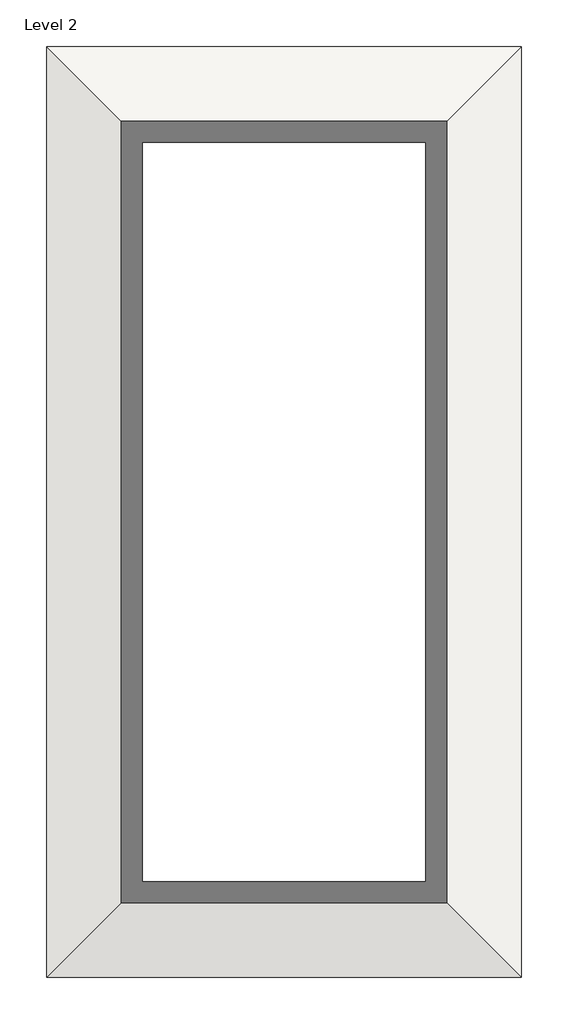
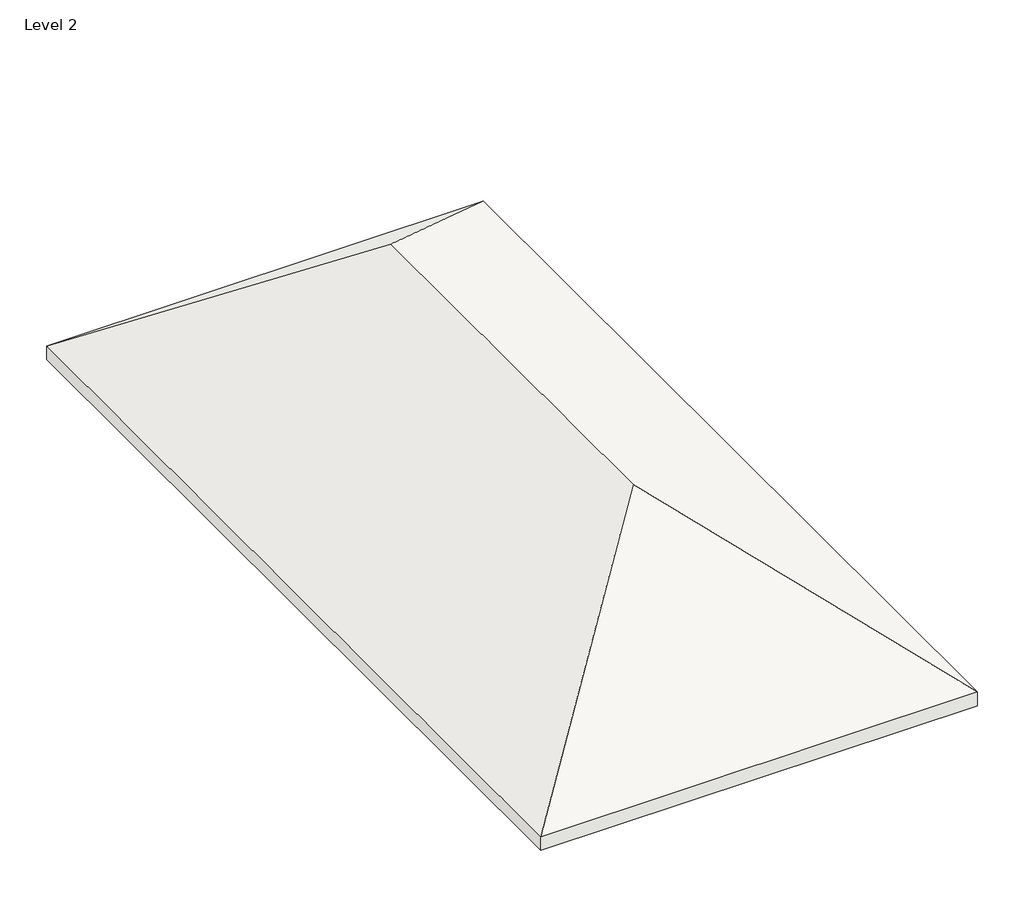
# One storey: 1 roof.
"""IFC4 building model written with IfcOpenShell, lengths in millimetres."""

from ifc_helpers import new_model, si_unit, origin, place, context, project, spatial, faceted_brep, element, save

model = new_model("IFC4")

# Units and contexts
model_context = context("Model", 3, world=origin())
ifc_project = project(units=[si_unit("LENGTHUNIT", "METRE", prefix="MILLI")], contexts=[model_context])

# Site, building, storey
site = spatial("IfcSite", under=ifc_project)
building = spatial("IfcBuilding", under=site)
storey = spatial("IfcBuildingStorey", under=building, Name="Level 2", Elevation=3048.0)

# Roof
placement = place(None, origin())
element("IfcRoof", 1, ObjectType="Wood Rafter 8\" - Asphalt Shingle - Insulated", at=placement, inside=storey, context=model_context, shape_type="Brep", body=[
    faceted_brep([(-269.7374913, 11860.1394299, 3048.0), (-4221.0249913, 7908.8519299, 6011.465625), (-8172.3124913, 11860.1394299, 3048.0), (-4221.0249913, 320.6019299, 6011.465625), (-8172.3124913, -3630.6855701, 3048.0), (-269.7374913, -3630.6855701, 3048.0), (-269.7374913, 11860.1394299, 3313.90625), (-8172.3124913, 11860.1394299, 3313.90625), (-4221.0249913, 7908.8519299, 6277.371875), (-8172.3124913, -3630.6855701, 3313.90625), (-4221.0249913, 320.6019299, 6277.371875), (-269.7374913, -3630.6855701, 3313.90625)], [[[0, 1, 2]], [[2, 1, 3, 4]], [[4, 3, 5]], [[1, 0, 5, 3]], [[6, 7, 8]], [[7, 9, 10, 8]], [[9, 11, 10]], [[6, 8, 10, 11]], [[2, 7, 6, 0]], [[4, 9, 7, 2]], [[5, 11, 9, 4]], [[0, 6, 11, 5]]]),
])

save(model, "model.ifc")

# Revit data of these elements
# Type "Wood Rafter 8\" - Asphalt Shingle - Insulated"
#   Assembly Code = "B1020"
#   Layers, outside or top first: 0' - 0 1/4" "Asphalt Shingle" (function 4); 0' - 0 5/8" "Plywood, Sheathing" (function 2); 0' - 7 1/2" "Structure, Wood Joist/Rafter Layer, Batt Insulation" (function 1)
# Element 1 (IfcRoof, "Wood Rafter 8\" - Asphalt Shingle - Insulated")
#   built-in parameter 1001705 = 20.5951 (stored number, unit not read)
#   built-in parameter 1001710 = 33615
#   Phase Created = New Construction
#   Materials on its faces: "Structure, Wood Joist/Rafter Layer, Batt Insulation", "Asphalt Shingle"
# Materials
#   "Asphalt Shingle": class "Generic", colour RGB 155 155 155, transparency 0, Description = "Asphalt roofing shingle", Cost = 0
#   "Plywood, Sheathing": class "Wood", colour RGB 212 179 113, transparency 0, Description = "Plywood, sheathing grade", Cost = 0
#   "Structure, Wood Joist/Rafter Layer, Batt Insulation": class "Wood", colour RGB 127 127 127, transparency 0, Description = "Wood framing, insulated", Cost = 0
